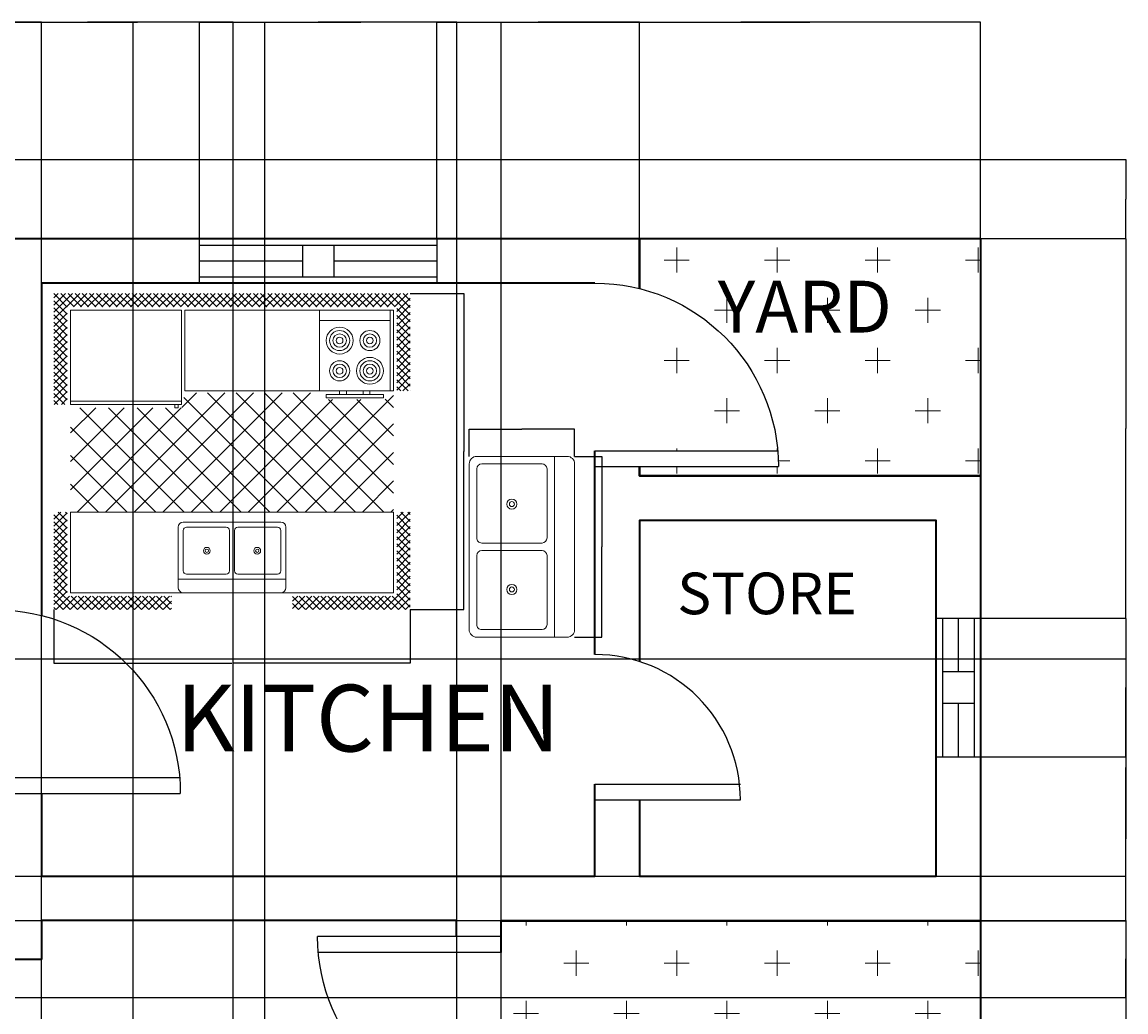
# Model space of a CAD drawing. Units: millimetres. Extents: x 19292 to 100733, y 12374 to 26974.
# Tile 18 of 24: x 31296 to 36880, y 18550 to 23556. Entities that reach past the tile are written whole.
import ezdxf

# ---------------------------------------------------------------- set-up
doc = ezdxf.new("R2010")
doc.units = ezdxf.units.MM
for name, color, linetype, lineweight in [('A-ANNO-DIMS', 2, 'Continuous', 18), ('A-AREA-IDEN', 3, 'Continuous', 25), ('A-DOOR', 4, 'Continuous', 25), ('A-FLOR-FIXT', 9, 'Continuous', 18), ('A-FLOR-PATT', 252, 'Continuous', 13), ('A-GLAZ', 3, 'Continuous', 25), ('A-WALL', 7, 'Continuous', 35)]:
    doc.layers.add(name, color=color, linetype=linetype, lineweight=lineweight)
doc.layers.add('WINDOWS', color=50, linetype='Continuous')
doc.styles.get("Standard").update_dxf_attribs({"font": 'arial.ttf'})
doc.dimstyles.get("Standard").update_dxf_attribs({"dimtxt": 0.18, "dimasz": 0.18, "dimexe": 0.18, "dimexo": 0.0625, "dimgap": 0.09, "dimtad": 0, "dimtih": 1, "dimtoh": 1, "dimdec": 4, "dimzin": 0, "dimdsep": 46, "dimtxsty": 'Standard', "dimcen": 0.09, "dimadec": 0, "dimazin": 0, "dimtfac": 1, "dimtdec": 4, "dimtofl": 0, "dimtmove": 0, "dimatfit": 3, "dimfxl": 1, "dimtolj": 1, "dimtzin": 0, "dimarcsym": 0})

# ---------------------------------------------------------------- blocks, each defined once
blk = doc.blocks.new('WW34')
at = {"layer": 'WINDOWS'}
for p, q in [((6711.3, 3446), (7411.3, 3446)), ((6981.3, 3446), (6981.3, 3286)), ((7141.3, 3446), (7141.3, 3286)), ((6711.3, 3366), (6981.3, 3366)), ((7141.3, 3366), (7411.3, 3366)), ((6711.3, 3286), (7411.3, 3286))]:
    blk.add_line(p, q, dxfattribs=at)
for points in [[(6711.3, 3478.5), (6711.3, 3253.5)], [(7411.3, 3253.5), (7411.3, 3478.5)]]:
    blk.add_lwpolyline(points, dxfattribs=at)
blk = doc.blocks.new('WW')
at = {"layer": 'WINDOWS'}
for p, q in [((-5183.9, -4940.9), (-3983.9, -4940.9)), ((-4663.9, -4940.9), (-4663.9, -5100.9)), ((-4503.9, -4940.9), (-4503.9, -5100.9)), ((-4503.9, -4940.9), (-4503.9, -5100.9)), ((-5183.9, -5020.9), (-4663.9, -5020.9)), ((-4503.9, -5020.9), (-3983.9, -5020.9)), ((-5183.9, -5100.9), (-3983.9, -5100.9))]:
    blk.add_line(p, q, dxfattribs=at)
for points in [[(-5183.9, -5133.4), (-5183.9, -4908.4)], [(-3983.9, -4908.4), (-3983.9, -5133.4)]]:
    blk.add_lwpolyline(points, dxfattribs=at)
blk = doc.blocks.new('Kitchen Layout - 7 x 8 ft')
for p, q in [((-5, 81.32), (2.68, 89)), ((-5, 83.44), (0.56, 89)), ((-5, 85.56), (-1.56, 89)), ((-5, 87.68), (-3.68, 89)), ((-1, 84.97), (-5, 88.97)), ((1.09, 85), (-2.91, 89)), ((3.21, 85), (-0.79, 89)), ((0.81, 85), (4.81, 89)), ((5.34, 85), (1.34, 89)), ((2.93, 85), (6.93, 89)), ((7.46, 85), (3.46, 89)), ((5.05, 85), (9.05, 89)), ((9.58, 85), (5.58, 89)), ((7.17, 85), (11.17, 89)), ((11.7, 85), (7.7, 89)), ((9.29, 85), (13.29, 89)), ((13.82, 85), (9.82, 89)), ((11.41, 85), (15.41, 89)), ((15.94, 85), (11.94, 89)), ((13.53, 85), (17.53, 89)), ((18.06, 85), (14.06, 89)), ((15.65, 85), (19.65, 89)), ((20.18, 85), (16.18, 89)), ((17.78, 85), (21.78, 89)), ((22.31, 85), (18.31, 89)), ((19.9, 85), (23.9, 89)), ((24.43, 85), (20.43, 89)), ((22.02, 85), (26.02, 89)), ((26.55, 85), (22.55, 89)), ((24.14, 85), (28.14, 89)), ((28.67, 85), (24.67, 89)), ((26.26, 85), (30.26, 89)), ((30.79, 85), (26.79, 89)), ((28.38, 85), (32.38, 89)), ((32.91, 85), (28.91, 89)), ((30.5, 85), (34.5, 89)), ((35.03, 85), (31.03, 89)), ((32.63, 85), (36.63, 89)), ((37.16, 85), (33.16, 89)), ((34.75, 85), (38.75, 89)), ((39.28, 85), (35.28, 89)), ((36.87, 85), (40.87, 89)), ((41.4, 85), (37.4, 89)), ((38.99, 85), (42.99, 89)), ((43.52, 85), (39.52, 89)), ((41.11, 85), (45.11, 89)), ((45.64, 85), (41.64, 89)), ((43.23, 85), (47.23, 89)), ((47.76, 85), (43.76, 89)), ((45.35, 85), (49.35, 89)), ((49.88, 85), (45.88, 89)), ((47.47, 85), (51.47, 89)), ((52, 85), (48, 89)), ((49.6, 85), (53.6, 89)), ((54.13, 85), (50.13, 89)), ((51.72, 85), (55.72, 89)), ((56.25, 85), (52.25, 89)), ((53.84, 85), (57.84, 89)), ((58.37, 85), (54.37, 89)), ((55.96, 85), (59.96, 89)), ((60.49, 85), (56.49, 89)), ((58.08, 85), (62.08, 89)), ((62.61, 85), (58.61, 89)), ((60.2, 85), (64.2, 89)), ((64.73, 85), (60.73, 89)), ((62.32, 85), (66.32, 89)), ((66.85, 85), (62.85, 89)), ((64.45, 85), (68.45, 89)), ((68.97, 85), (64.97, 89)), ((66.57, 85), (70.57, 89)), ((71.1, 85), (67.1, 89)), ((68.69, 85), (72.69, 89)), ((73.22, 85), (69.22, 89)), ((70.81, 85), (74.81, 89)), ((75.34, 85), (71.34, 89)), ((72.93, 85), (76.93, 89)), ((77.46, 85), (73.46, 89)), ((75.05, 85), (79.05, 89)), ((79.58, 85), (75.58, 89)), ((77.17, 85), (81.17, 89)), ((81.7, 85), (77.7, 89)), ((79.29, 85), (83.29, 89)), ((83.82, 85), (79.82, 89)), ((81.42, 85), (85.42, 89)), ((85.95, 85), (81.95, 89)), ((83.54, 85), (87.54, 89)), ((88.07, 85), (84.07, 89)), ((85.66, 85), (89.66, 89)), ((90.19, 85), (86.19, 89)), ((87.78, 85), (91.78, 89)), ((92.31, 85), (88.31, 89)), ((89.9, 85), (93.9, 89)), ((94.43, 85), (90.43, 89)), ((92.02, 85), (96.02, 89)), ((96.55, 85), (92.55, 89)), ((94.14, 85), (98.14, 89)), ((101, 82.67), (94.67, 89)), ((96.27, 85), (100.27, 89)), ((101, 84.79), (96.79, 89)), ((101, 86.92), (98.92, 89)), ((-1, 82.85), (-5, 86.85)), ((97, 83.61), (101, 87.61)), ((97, 81.49), (101, 85.49)), ((-1, 80.73), (-5, 84.73)), ((-5, 79.19), (-1, 83.19)), ((-1, 78.61), (-5, 82.61)), ((34, 84), (96, 84)), ((34, 60), (34, 84)), ((96, 84), (96, 60)), ((101, 80.55), (97, 84.55)), ((97, 79.37), (101, 83.37)), ((101, 78.43), (97, 82.43)), ((-5, 77.07), (-1, 81.07)), ((-1, 76.49), (-5, 80.49)), ((-5, 74.95), (-1, 78.95)), ((74, 81), (95, 81)), ((97, 77.25), (101, 81.25)), ((101, 76.31), (97, 80.31)), ((97, 75.13), (101, 79.13)), ((-1, 74.36), (-5, 78.36)), ((-5, 72.83), (-1, 76.83)), ((-1, 72.24), (-5, 76.24)), ((101, 74.19), (97, 78.19)), ((97, 73.01), (101, 77.01)), ((101, 72.07), (97, 76.07)), ((-5, 70.71), (-1, 74.71)), ((-1, 70.12), (-5, 74.12)), ((-5, 68.59), (-1, 72.59)), ((97, 70.89), (101, 74.89)), ((101, 69.95), (97, 73.95)), ((97, 68.76), (101, 72.76)), ((-1, 68), (-5, 72)), ((-5, 66.47), (-1, 70.47)), ((-1, 65.88), (-5, 69.88)), ((101, 67.82), (97, 71.82)), ((97, 66.64), (101, 70.64)), ((101, 65.7), (97, 69.7)), ((-5, 64.35), (-1, 68.35)), ((-1, 63.76), (-5, 67.76)), ((-5, 62.22), (-1, 66.22)), ((97, 64.52), (101, 68.52)), ((101, 63.58), (97, 67.58)), ((97, 62.4), (101, 66.4)), ((-1, 61.64), (-5, 65.64)), ((-5, 60.1), (-1, 64.1)), ((-1, 59.52), (-5, 63.52)), ((101, 61.46), (97, 65.46)), ((97, 60.28), (101, 64.28)), ((100.34, 60), (97, 63.34)), ((-5, 57.98), (-1, 61.98)), ((-1, 57.39), (-5, 61.39)), ((-1.73, 56), (-5, 59.27)), ((-4.86, 56), (-1, 59.86)), ((10.4, 24), (45.9, 59.5)), ((18.88, 24), (54.38, 59.5)), ((27.37, 24), (62.87, 59.5)), ((33.03, 55.11), (37.41, 59.5)), ((96, 60), (34, 60)), ((35.85, 24), (71.35, 59.5)), ((76.2, 24), (40.7, 59.5)), ((84.68, 24), (49.18, 59.5)), ((93.17, 24), (57.67, 59.5)), ((96, 29.65), (66.15, 59.5)), ((80, 60), (80, 59)), ((82, 59), (82, 60)), ((87, 59), (87, 60)), ((89, 60), (89, 59)), ((98.22, 60), (97, 61.22)), ((98.84, 60), (101, 62.16)), ((100.96, 60), (101, 60.04)), ((-3.85, 56), (-5, 57.15)), ((-2.74, 56), (-1, 57.74)), ((0, 57), (33, 57)), ((31, 55), (31, 56)), ((32, 56), (32, 55)), ((67.71, 24), (33.68, 58.04)), ((44.34, 24), (77.84, 57.5)), ((52.82, 24), (86.32, 57.5)), ((61.31, 24), (96, 58.69)), ((96, 38.14), (76.64, 57.5)), ((96, 46.63), (85.13, 57.5)), ((96, 55.11), (93.57, 57.54)), ((0, 30.57), (24.43, 55)), ((0, 39.06), (15.94, 55)), ((0, 47.54), (7.46, 55)), ((1.91, 24), (32.91, 55)), ((33.77, 24), (2.77, 55)), ((42.26, 24), (11.26, 55)), ((50.74, 24), (19.74, 55)), ((59.23, 24), (28.23, 55)), ((32, 55), (31, 55)), ((25.29, 24), (0, 49.29)), ((69.79, 24), (96, 50.21)), ((16.8, 24), (0, 40.8)), ((78.28, 24), (96, 41.72)), ((86.76, 24), (96, 33.24)), ((8.32, 24), (0, 32.32)), ((-5, 21.92), (-2.92, 24)), ((-5, 19.8), (-1, 23.8)), ((-1, 19.21), (-5, 23.21)), ((-1, 21.33), (-3.67, 24)), ((-1, 23.45), (-1.55, 24)), ((0, 24), (96, 24)), ((0, 0), (0, 24)), ((95.25, 24), (96, 24.75)), ((96, 24), (96, 0)), ((97, 22.1), (98.9, 24)), ((97, 19.97), (101, 23.97)), ((101, 19.03), (97, 23.03)), ((101, 21.16), (98.16, 24)), ((101, 23.28), (100.28, 24)), ((-5, 17.68), (-1, 21.68)), ((-1, 17.09), (-5, 21.09)), ((97, 17.85), (101, 21.85)), ((101, 16.91), (97, 20.91)), ((97, 15.73), (101, 19.73)), ((-5, 15.55), (-1, 19.55)), ((-1, 14.97), (-5, 18.97)), ((-5, 13.43), (-1, 17.43)), ((-1, 12.85), (-5, 16.85)), ((47.25, 6.5), (47.25, 18.5)), ((48.75, 18.5), (48.75, 6.5)), ((101, 14.79), (97, 18.79)), ((97, 13.61), (101, 17.61)), ((101, 12.67), (97, 16.67)), ((-5, 11.31), (-1, 15.31)), ((-1, 10.73), (-5, 14.73)), ((-5, 9.19), (-1, 13.19)), ((97, 11.49), (101, 15.49)), ((101, 10.55), (97, 14.55)), ((97, 9.37), (101, 13.37)), ((-1, 8.6), (-5, 12.6)), ((-5, 7.07), (-1, 11.07)), ((-1, 6.48), (-5, 10.48)), ((101, 8.43), (97, 12.43)), ((97, 7.25), (101, 11.25)), ((101, 6.31), (97, 10.31)), ((-5, 4.95), (-1, 8.95)), ((-1, 4.36), (-5, 8.36)), ((-5, 2.83), (-1, 6.83)), ((97, 5.12), (101, 9.12)), ((101, 4.18), (97, 8.18)), ((97, 3), (101, 7)), ((-1, 2.24), (-5, 6.24)), ((-5, 0.71), (-1, 4.71)), ((-1, 0.12), (-5, 4.12)), ((64, 4), (32, 4)), ((101, 2.06), (97, 6.06)), ((97, 0.88), (101, 4.88)), ((101, -0.06), (97, 3.94)), ((-5, -1.42), (-1, 2.58)), ((2, -5), (-5, 2)), ((-5, -3.54), (-1, 0.46)), ((96, 0), (0, 0)), ((93.24, -5), (101, 2.76)), ((95.36, -5), (101, 0.64)), ((101, -2.18), (97, 1.82)), ((-0.12, -5), (-5, -0.12)), ((-2.25, -5), (-5, -2.25)), ((-4.34, -5), (-0.34, -1)), ((-2.22, -5), (1.78, -1)), ((-0.1, -5), (3.9, -1)), ((4.12, -5), (0.12, -1)), ((2.02, -5), (6.02, -1)), ((6.24, -5), (2.24, -1)), ((4.14, -5), (8.14, -1)), ((8.36, -5), (4.36, -1)), ((6.27, -5), (10.27, -1)), ((10.48, -5), (6.48, -1)), ((8.39, -5), (12.39, -1)), ((12.6, -5), (8.6, -1)), ((10.51, -5), (14.51, -1)), ((14.73, -5), (10.73, -1)), ((12.63, -5), (16.63, -1)), ((16.85, -5), (12.85, -1)), ((14.75, -5), (18.75, -1)), ((18.97, -5), (14.97, -1)), ((16.87, -5), (20.87, -1)), ((21.09, -5), (17.09, -1)), ((18.99, -5), (22.99, -1)), ((23.21, -5), (19.21, -1)), ((21.11, -5), (25.11, -1)), ((25.33, -5), (21.33, -1)), ((23.24, -5), (27.24, -1)), ((27.45, -5), (23.45, -1)), ((25.36, -5), (29.36, -1)), ((29.57, -5), (25.57, -1)), ((27.48, -5), (30, -2.48)), ((30, -3.3), (27.7, -1)), ((30, -1.18), (29.82, -1)), ((66, -2.54), (67.54, -1)), ((66, -4.66), (69.66, -1)), ((69.88, -5), (66, -1.12)), ((67.76, -5), (66, -3.24)), ((67.78, -5), (71.78, -1)), ((72, -5), (68, -1)), ((69.9, -5), (73.9, -1)), ((74.12, -5), (70.12, -1)), ((72.03, -5), (76.03, -1)), ((76.24, -5), (72.24, -1)), ((74.15, -5), (78.15, -1)), ((78.36, -5), (74.36, -1)), ((76.27, -5), (80.27, -1)), ((80.49, -5), (76.49, -1)), ((78.39, -5), (82.39, -1)), ((82.61, -5), (78.61, -1)), ((80.51, -5), (84.51, -1)), ((84.73, -5), (80.73, -1)), ((82.63, -5), (86.63, -1)), ((86.85, -5), (82.85, -1)), ((84.75, -5), (88.75, -1)), ((88.97, -5), (84.97, -1)), ((86.88, -5), (90.88, -1)), ((91.09, -5), (87.09, -1)), ((89, -5), (93, -1)), ((93.21, -5), (89.21, -1)), ((91.12, -5), (95.12, -1)), ((95.34, -5), (91.34, -1)), ((97.46, -5), (93.46, -1)), ((99.58, -5), (95.58, -1)), ((101, -4.3), (97, -0.3)), ((97.48, -5), (101, -1.48)), ((-4.37, -5), (-5, -4.37)), ((29.6, -5), (30, -4.6)), ((99.6, -5), (101, -3.6))]:
    blk.add_line(p, q)
for points in [[(0, 56), (0, 84), (33, 84), (33, 56)], [(74, 60), (74, 84), (95, 84), (95, 60)], [(76, 58), (76, 59), (93, 59), (93, 58)]]:
    blk.add_lwpolyline(points, close=True)
for points in [[(33.5, 21), (62.5, 21)], [(32, 1.5), (32, 19.5)], [(33.5, 6.5), (33.5, 18.5)], [(34.5, 19.5), (46.25, 19.5)], [(49.75, 19.5), (61.5, 19.5)], [(62.5, 18.5), (62.5, 6.5)], [(64, 19.5), (64, 1.5)], [(46.25, 5.5), (34.5, 5.5)], [(61.5, 5.5), (49.75, 5.5)], [(62.5, 0), (33.5, 0)]]:
    blk.add_lwpolyline(points)
for centre, radius in [((80, 75), 4), ((80, 75), 3), ((80, 75), 2), ((80, 75), 1), ((89, 75), 3), ((89, 75), 2), ((89, 75), 1), ((80, 66), 3), ((89, 66), 4), ((89, 66), 3), ((80, 66), 2), ((80, 66), 1), ((89, 66), 2), ((89, 66), 1), ((40.5, 12.5), 1), ((55.5, 12.5), 1), ((40.5, 12.5), 0.5), ((55.5, 12.5), 0.5)]:
    blk.add_circle(centre, radius)
for centre, radius, start, end in [((33.5, 19.5), 1.5, 90, 180), ((62.5, 19.5), 1.5, 0, 90), ((34.5, 18.5), 1, 90, 180), ((46.25, 18.5), 1, 0, 90), ((49.75, 18.5), 1, 90, 180), ((61.5, 18.5), 1, 0, 90), ((34.5, 6.5), 1, 180, 270), ((46.25, 6.5), 1, 270, 0), ((49.75, 6.5), 1, 180, 270), ((61.5, 6.5), 1, 270, 0), ((33.5, 1.5), 1.5, 180, 270), ((62.5, 1.5), 1.5, 270, 0)]:
    blk.add_arc(centre, radius, start, end)
blk = doc.blocks.new('Sink-double - 36 in top')
for p, q in [((-18, -4), (18, -4)), ((-0.75, -18.5), (-0.75, -6.5)), ((0.75, -6.5), (0.75, -18.5))]:
    blk.add_line(p, q)
for points in [[(-16.5, 0), (16.5, 0)], [(-18, -19.5), (-18, -1.5)], [(18, -1.5), (18, -19.5)], [(-16.5, -18.5), (-16.5, -6.5)], [(-15.5, -5.5), (-1.75, -5.5)], [(1.75, -5.5), (15.5, -5.5)], [(16.5, -6.5), (16.5, -18.5)], [(-1.75, -19.5), (-15.5, -19.5)], [(15.5, -19.5), (1.75, -19.5)], [(16.5, -21), (-16.5, -21)]]:
    blk.add_lwpolyline(points)
for centre, radius in [((-8.5, -12.5), 1), ((-8.5, -12.5), 0.5), ((8.5, -12.5), 1), ((8.5, -12.5), 0.5)]:
    blk.add_circle(centre, radius)
for centre, radius, start, end in [((-16.5, -1.5), 1.5, 90, 180), ((16.5, -1.5), 1.5, 0, 90), ((-15.5, -6.5), 1, 90, 180), ((-1.75, -6.5), 1, 0, 90), ((1.75, -6.5), 1, 90, 180), ((15.5, -6.5), 1, 0, 90), ((-16.5, -19.5), 1.5, 180, 270), ((-15.5, -18.5), 1, 180, 270), ((-1.75, -18.5), 1, 270, 0), ((1.75, -18.5), 1, 180, 270), ((15.5, -18.5), 1, 270, 0), ((16.5, -19.5), 1.5, 270, 0)]:
    blk.add_arc(centre, radius, start, end)
blk = doc.blocks.new('DOOR-900')
for p, q in [((927.7, 80), (0, 80)), ((927.7, 0), (927.7, 80)), ((927.7, 0), (927.7, 80)), ((927.7, 0), (0, 0))]:
    blk.add_line(p, q)
blk.add_arc((927.7, 0), 927.7, 90, 180)
blk = doc.blocks.new('DOOR-SWING-900')
blk.add_line((927.7, 927.7), (927.7, 0))
blk.add_arc((927.7, 927.7), 927.7, 180, 270)
blk = doc.blocks.new('DOOR-SWING-750')
blk.add_line((0, 0), (735.3, 0))
blk.add_arc((0, 0), 735.3, 0, 90)
blk = doc.blocks.new('*D52')
at = {"layer": 'A-ANNO-DIMS', "color": 0, "lineweight": -2, "transparency": 16777216}
for p, q in [((31457.2, 20584.7), (31457.2, 20314.2)), ((33259.7, 20584.7), (33259.7, 20314.2)), ((31457.4, 20314.4), (32356.9, 20314.4)), ((33259.5, 20314.4), (32360.1, 20314.4))]:
    blk.add_line(p, q, dxfattribs=at)
at = {"layer": 'A-ANNO-DIMS', "color": 0, "transparency": 16777216}
for points in [[(31457.4, 20314.5), (31457.4, 20314.4), (31457.2, 20314.4)], [(33259.5, 20314.5), (33259.5, 20314.4), (33259.7, 20314.4)]]:
    blk.add_solid(points, dxfattribs=at)
at = {"layer": 'Defpoints', "color": 0, "transparency": 16777216}
for p in [(31457.2, 20584.8), (33259.7, 20584.8), (33259.7, 20314.4)]:
    blk.add_point(p, dxfattribs=at)
at = {"layer": 'A-ANNO-DIMS', "color": 0, "transparency": 16777216, "insert": (32358.5, 20314.4), "char_height": 0.18, "attachment_point": 5}
blk.add_mtext('\\A1;KITCHEN COUNTER 1803', dxfattribs=at)
blk = doc.blocks.new('*D53')
at = {"layer": 'A-ANNO-DIMS', "color": 0, "lineweight": -2, "transparency": 16777216}
for p, q in [((33259.8, 22183.3), (33530.3, 22183.3)), ((33530.1, 22183.1), (33530.1, 21384.2)), ((33530.1, 20585), (33530.1, 21383.9)), ((33259.8, 20584.8), (33530.3, 20584.8))]:
    blk.add_line(p, q, dxfattribs=at)
at = {"layer": 'A-ANNO-DIMS', "color": 0, "transparency": 16777216}
for points in [[(33530.1, 22183.1), (33530.1, 22183.1), (33530.1, 22183.3)], [(33530.1, 20585), (33530.1, 20585), (33530.1, 20584.8)]]:
    blk.add_solid(points, dxfattribs=at)
at = {"layer": 'Defpoints', "color": 0, "transparency": 16777216}
for p in [(33259.7, 22183.3), (33530.1, 22183.3), (33259.7, 20584.8)]:
    blk.add_point(p, dxfattribs=at)
at = {"layer": 'A-ANNO-DIMS', "color": 0, "transparency": 16777216, "insert": (33530.1, 21384), "char_height": 0.18, "attachment_point": 5}
blk.add_mtext('\\A1;1598', dxfattribs=at)
blk = doc.blocks.new('*D54')
at = {"layer": 'A-ANNO-DIMS', "color": 0, "lineweight": -2, "transparency": 16777216}
for p, q in [((34091.3, 21359.4), (34228.6, 21359.4)), ((34228.4, 21359.2), (34228.4, 20902.4)), ((34228.4, 20445.2), (34228.4, 20902)), ((34091.3, 20445), (34228.6, 20445))]:
    blk.add_line(p, q, dxfattribs=at)
at = {"layer": 'A-ANNO-DIMS', "color": 0, "transparency": 16777216}
for points in [[(34228.4, 21359.2), (34228.5, 21359.2), (34228.4, 21359.4)], [(34228.4, 20445.2), (34228.5, 20445.2), (34228.4, 20445)]]:
    blk.add_solid(points, dxfattribs=at)
at = {"layer": 'Defpoints', "color": 0, "transparency": 16777216}
for p in [(34091.3, 21359.4), (34091.3, 20445), (34228.4, 20445)]:
    blk.add_point(p, dxfattribs=at)
at = {"layer": 'A-ANNO-DIMS', "color": 0, "transparency": 16777216, "insert": (34228.4, 20902.2), "char_height": 0.18, "attachment_point": 5}
blk.add_mtext('\\A1;DOUBLE SINK 914', dxfattribs=at)
blk = doc.blocks.new('*D55')
at = {"layer": 'A-ANNO-DIMS', "color": 0, "lineweight": -2, "transparency": 16777216}
for p, q in [((33557.9, 21359.5), (33557.9, 21496.8)), ((33558, 21496.6), (33824.3, 21496.6)), ((34091.1, 21496.6), (33824.9, 21496.6)), ((34091.3, 21359.5), (34091.3, 21496.8))]:
    blk.add_line(p, q, dxfattribs=at)
at = {"layer": 'A-ANNO-DIMS', "color": 0, "transparency": 16777216}
for points in [[(33558, 21496.6), (33558, 21496.5), (33557.9, 21496.6)], [(34091.1, 21496.6), (34091.1, 21496.5), (34091.3, 21496.6)]]:
    blk.add_solid(points, dxfattribs=at)
at = {"layer": 'Defpoints', "color": 0, "transparency": 16777216}
for p in [(34091.3, 21496.6), (33557.9, 21359.4), (34091.3, 21359.4)]:
    blk.add_point(p, dxfattribs=at)
at = {"layer": 'A-ANNO-DIMS', "color": 0, "transparency": 16777216, "insert": (33824.6, 21496.6), "char_height": 0.18, "attachment_point": 5}
blk.add_mtext('\\A1;533', dxfattribs=at)
blk = doc.blocks.new('*D63')
at = {"layer": 'A-ANNO-DIMS', "color": 0, "lineweight": -2, "transparency": 16777216}
for p, q in [((31169.1, 22460.8), (31169.1, 23555.9)), ((31169.3, 23555.7), (31681.3, 23555.7)), ((32194, 23555.7), (31682, 23555.7)), ((32194.1, 22460.8), (32194.1, 23555.9))]:
    blk.add_line(p, q, dxfattribs=at)
at = {"layer": 'A-ANNO-DIMS', "color": 0, "transparency": 16777216}
for points in [[(31169.3, 23555.8), (31169.3, 23555.7), (31169.1, 23555.7)], [(32194, 23555.8), (32194, 23555.7), (32194.1, 23555.7)]]:
    blk.add_solid(points, dxfattribs=at)
at = {"layer": 'Defpoints', "color": 0, "transparency": 16777216}
for p in [(32194.1, 23555.7), (31169.1, 22460.7), (32194.1, 22460.7)]:
    blk.add_point(p, dxfattribs=at)
at = {"layer": 'A-ANNO-DIMS', "color": 0, "transparency": 16777216, "insert": (31681.6, 23555.7), "char_height": 0.18, "attachment_point": 5}
blk.add_mtext('\\A1;1025', dxfattribs=at)
blk = doc.blocks.new('*D64')
at = {"layer": 'A-ANNO-DIMS', "color": 0, "lineweight": -2, "transparency": 16777216}
for p, q in [((32194.1, 22460.8), (32194.1, 23555.9)), ((32194.3, 23555.7), (32793.8, 23555.7)), ((33394, 23555.7), (32794.5, 23555.7)), ((33394.1, 22460.8), (33394.1, 23555.9))]:
    blk.add_line(p, q, dxfattribs=at)
at = {"layer": 'A-ANNO-DIMS', "color": 0, "transparency": 16777216}
for points in [[(32194.3, 23555.8), (32194.3, 23555.7), (32194.1, 23555.7)], [(33394, 23555.8), (33394, 23555.7), (33394.1, 23555.7)]]:
    blk.add_solid(points, dxfattribs=at)
at = {"layer": 'Defpoints', "color": 0, "transparency": 16777216}
for p in [(33394.1, 23555.7), (32194.1, 22460.7), (33394.1, 22460.7)]:
    blk.add_point(p, dxfattribs=at)
at = {"layer": 'A-ANNO-DIMS', "color": 0, "transparency": 16777216, "insert": (32794.1, 23555.7), "char_height": 0.18, "attachment_point": 5}
blk.add_mtext('\\A1;1200', dxfattribs=at)
blk = doc.blocks.new('*D65')
at = {"layer": 'A-ANNO-DIMS', "color": 0, "lineweight": -2, "transparency": 16777216}
for p, q in [((33394.1, 22460.8), (33394.1, 23555.9)), ((33394.3, 23555.7), (33906.3, 23555.7)), ((34419, 23555.7), (33907, 23555.7)), ((34419.1, 22460.8), (34419.1, 23555.9))]:
    blk.add_line(p, q, dxfattribs=at)
at = {"layer": 'A-ANNO-DIMS', "color": 0, "transparency": 16777216}
for points in [[(33394.3, 23555.8), (33394.3, 23555.7), (33394.1, 23555.7)], [(34419, 23555.8), (34419, 23555.7), (34419.1, 23555.7)]]:
    blk.add_solid(points, dxfattribs=at)
at = {"layer": 'Defpoints', "color": 0, "transparency": 16777216}
for p in [(34419.1, 23555.7), (33394.1, 22460.7), (34419.1, 22460.7)]:
    blk.add_point(p, dxfattribs=at)
at = {"layer": 'A-ANNO-DIMS', "color": 0, "transparency": 16777216, "insert": (33906.6, 23555.7), "char_height": 0.18, "attachment_point": 5}
blk.add_mtext('\\A1;1025', dxfattribs=at)
blk = doc.blocks.new('*D66')
at = {"layer": 'A-ANNO-DIMS', "color": 0, "lineweight": -2, "transparency": 16777216}
for p, q in [((34419.1, 22460.8), (34419.1, 23555.9)), ((34419.3, 23555.7), (35281.3, 23555.7)), ((36144, 23555.7), (35282, 23555.7)), ((36144.1, 22460.8), (36144.1, 23555.9))]:
    blk.add_line(p, q, dxfattribs=at)
at = {"layer": 'A-ANNO-DIMS', "color": 0, "transparency": 16777216}
for points in [[(34419.3, 23555.8), (34419.3, 23555.7), (34419.1, 23555.7)], [(36144, 23555.8), (36144, 23555.7), (36144.1, 23555.7)]]:
    blk.add_solid(points, dxfattribs=at)
at = {"layer": 'Defpoints', "color": 0, "transparency": 16777216}
for p in [(36144.1, 23555.7), (34419.1, 22460.7), (36144.1, 22460.7)]:
    blk.add_point(p, dxfattribs=at)
at = {"layer": 'A-ANNO-DIMS', "color": 0, "transparency": 16777216, "insert": (35281.6, 23555.7), "char_height": 0.18, "attachment_point": 5}
blk.add_mtext('\\A1;1725', dxfattribs=at)
blk = doc.blocks.new('*D68')
at = {"layer": 'A-ANNO-DIMS', "color": 0, "lineweight": -2, "transparency": 16777216}
for p, q in [((22919.2, 20335.7), (36879.3, 20335.7)), ((36879.2, 20335.5), (36879.2, 19785.9)), ((36879.2, 19235.9), (36879.2, 19785.5)), ((22919.2, 19235.7), (36879.3, 19235.7))]:
    blk.add_line(p, q, dxfattribs=at)
at = {"layer": 'A-ANNO-DIMS', "color": 0, "transparency": 16777216}
for points in [[(36879.1, 20335.5), (36879.2, 20335.5), (36879.2, 20335.7)], [(36879.1, 19235.9), (36879.2, 19235.9), (36879.2, 19235.7)]]:
    blk.add_solid(points, dxfattribs=at)
at = {"layer": 'Defpoints', "color": 0, "transparency": 16777216}
for p in [(22919.1, 20335.7), (22919.1, 19235.7), (36879.2, 19235.7)]:
    blk.add_point(p, dxfattribs=at)
at = {"layer": 'A-ANNO-DIMS', "color": 0, "transparency": 16777216, "insert": (36879.2, 19785.7), "char_height": 0.18, "attachment_point": 5}
blk.add_mtext('\\A1;1100', dxfattribs=at)
blk = doc.blocks.new('*D69')
at = {"layer": 'A-ANNO-DIMS', "color": 0, "lineweight": -2, "transparency": 16777216}
for p, q in [((23573.9, 19012.7), (36879.3, 19012.7)), ((36879.2, 19012.6), (36879.2, 18818)), ((36879.2, 18623), (36879.2, 18817.6)), ((23573.9, 18622.9), (36879.3, 18622.9))]:
    blk.add_line(p, q, dxfattribs=at)
at = {"layer": 'A-ANNO-DIMS', "color": 0, "transparency": 16777216}
for points in [[(36879.1, 19012.6), (36879.2, 19012.6), (36879.2, 19012.7)], [(36879.1, 18623), (36879.2, 18623), (36879.2, 18622.9)]]:
    blk.add_solid(points, dxfattribs=at)
at = {"layer": 'Defpoints', "color": 0, "transparency": 16777216}
for p in [(23573.8, 19012.7), (23573.8, 18622.9), (36879.2, 18622.9)]:
    blk.add_point(p, dxfattribs=at)
at = {"layer": 'A-ANNO-DIMS', "color": 0, "transparency": 16777216, "insert": (36879.2, 18817.8), "char_height": 0.18, "attachment_point": 5}
blk.add_mtext('\\A1;389.9', dxfattribs=at)
blk = doc.blocks.new('*D74')
at = {"layer": 'A-ANNO-DIMS', "color": 0, "lineweight": -2, "transparency": 16777216}
for p, q in [((36144.2, 19010.7), (36879.3, 19010.7)), ((36879.2, 19010.5), (36879.2, 17498.4)), ((36879.2, 15985.9), (36879.2, 17498)), ((36144.2, 15985.7), (36879.3, 15985.7))]:
    blk.add_line(p, q, dxfattribs=at)
at = {"layer": 'A-ANNO-DIMS', "color": 0, "transparency": 16777216}
for points in [[(36879.1, 19010.5), (36879.2, 19010.5), (36879.2, 19010.7)], [(36879.1, 15985.9), (36879.2, 15985.9), (36879.2, 15985.7)]]:
    blk.add_solid(points, dxfattribs=at)
at = {"layer": 'Defpoints', "color": 0, "transparency": 16777216}
for p in [(36144.2, 19010.7), (36879.2, 19010.7), (36144.2, 15985.7)]:
    blk.add_point(p, dxfattribs=at)
at = {"layer": 'A-ANNO-DIMS', "color": 0, "transparency": 16777216, "insert": (36879.2, 17498.2), "char_height": 0.18, "attachment_point": 5}
blk.add_mtext('\\A1;3025', dxfattribs=at)
blk = doc.blocks.new('*D75')
at = {"layer": 'A-ANNO-DIMS', "color": 0, "lineweight": -2, "transparency": 16777216}
for p, q in [((36144.2, 19840.4), (36879.3, 19840.4)), ((36879.2, 19840.2), (36879.2, 19425.7)), ((36879.2, 19010.9), (36879.2, 19425.4)), ((36144.2, 19010.7), (36879.3, 19010.7))]:
    blk.add_line(p, q, dxfattribs=at)
at = {"layer": 'A-ANNO-DIMS', "color": 0, "transparency": 16777216}
for points in [[(36879.1, 19840.2), (36879.2, 19840.2), (36879.2, 19840.4)], [(36879.1, 19010.9), (36879.2, 19010.9), (36879.2, 19010.7)]]:
    blk.add_solid(points, dxfattribs=at)
at = {"layer": 'Defpoints', "color": 0, "transparency": 16777216}
for p in [(36144.1, 19840.4), (36879.2, 19840.4), (36144.2, 19010.7)]:
    blk.add_point(p, dxfattribs=at)
at = {"layer": 'A-ANNO-DIMS', "color": 0, "transparency": 16777216, "insert": (36879.2, 19425.6), "char_height": 0.18, "attachment_point": 5}
blk.add_mtext('\\A1;829.7', dxfattribs=at)
blk = doc.blocks.new('*D76')
at = {"layer": 'A-ANNO-DIMS', "color": 0, "lineweight": -2, "transparency": 16777216}
for p, q in [((36144.2, 20540.4), (36879.3, 20540.4)), ((36879.2, 20540.2), (36879.2, 20190.6)), ((36879.2, 19840.6), (36879.2, 20190.2)), ((36144.2, 19840.4), (36879.3, 19840.4))]:
    blk.add_line(p, q, dxfattribs=at)
at = {"layer": 'A-ANNO-DIMS', "color": 0, "transparency": 16777216}
for points in [[(36879.1, 20540.2), (36879.2, 20540.2), (36879.2, 20540.4)], [(36879.1, 19840.6), (36879.2, 19840.6), (36879.2, 19840.4)]]:
    blk.add_solid(points, dxfattribs=at)
at = {"layer": 'Defpoints', "color": 0, "transparency": 16777216}
for p in [(36144.1, 20540.4), (36879.2, 20540.4), (36144.1, 19840.4)]:
    blk.add_point(p, dxfattribs=at)
at = {"layer": 'A-ANNO-DIMS', "color": 0, "transparency": 16777216, "insert": (36879.2, 20190.4), "char_height": 0.18, "attachment_point": 5}
blk.add_mtext('\\A1;700', dxfattribs=at)
blk = doc.blocks.new('*D77')
at = {"layer": 'A-ANNO-DIMS', "color": 0, "lineweight": -2, "transparency": 16777216}
for p, q in [((36144.2, 22460.7), (36879.3, 22460.7)), ((36879.2, 22460.5), (36879.2, 21500.7)), ((36879.2, 20540.6), (36879.2, 21500.4)), ((36144.2, 20540.4), (36879.3, 20540.4))]:
    blk.add_line(p, q, dxfattribs=at)
at = {"layer": 'A-ANNO-DIMS', "color": 0, "transparency": 16777216}
for points in [[(36879.1, 22460.5), (36879.2, 22460.5), (36879.2, 22460.7)], [(36879.1, 20540.6), (36879.2, 20540.6), (36879.2, 20540.4)]]:
    blk.add_solid(points, dxfattribs=at)
at = {"layer": 'Defpoints', "color": 0, "transparency": 16777216}
for p in [(36144.1, 22460.7), (36879.2, 22460.7), (36144.1, 20540.4)]:
    blk.add_point(p, dxfattribs=at)
at = {"layer": 'A-ANNO-DIMS', "color": 0, "transparency": 16777216, "insert": (36879.2, 21500.6), "char_height": 0.18, "attachment_point": 5}
blk.add_mtext('\\A1;1920.3', dxfattribs=at)
blk = doc.blocks.new('*D78')
at = {"layer": 'A-ANNO-DIMS', "color": 0, "lineweight": -2, "transparency": 16777216}
for p, q in [((28369.2, 22860.7), (36879.3, 22860.7)), ((36879.2, 22860.5), (36879.2, 22660.9)), ((36879.2, 22460.9), (36879.2, 22660.5)), ((36144.2, 22460.7), (36879.3, 22460.7))]:
    blk.add_line(p, q, dxfattribs=at)
at = {"layer": 'A-ANNO-DIMS', "color": 0, "transparency": 16777216}
for points in [[(36879.1, 22860.5), (36879.2, 22860.5), (36879.2, 22860.7)], [(36879.1, 22460.9), (36879.2, 22460.9), (36879.2, 22460.7)]]:
    blk.add_solid(points, dxfattribs=at)
at = {"layer": 'Defpoints', "color": 0, "transparency": 16777216}
for p in [(28369.1, 22860.7), (36879.2, 22860.7), (36144.1, 22460.7)]:
    blk.add_point(p, dxfattribs=at)
at = {"layer": 'A-ANNO-DIMS', "color": 0, "transparency": 16777216, "insert": (36879.2, 22660.7), "char_height": 0.18, "attachment_point": 5}
blk.add_mtext('\\A1;400', dxfattribs=at)
blk = doc.blocks.new('*D79')
at = {"layer": 'A-ANNO-DIMS', "color": 0, "lineweight": -2, "transparency": 16777216}
for p, q in [((22694.1, 22860.7), (22694.1, 12808.8)), ((36144.2, 15985.7), (36144.2, 12808.8)), ((22694.3, 12809), (29418.7, 12809)), ((36144, 12809), (29419.6, 12809))]:
    blk.add_line(p, q, dxfattribs=at)
at = {"layer": 'A-ANNO-DIMS', "color": 0, "transparency": 16777216}
for points in [[(22694.3, 12809), (22694.3, 12809), (22694.1, 12809)], [(36144, 12809), (36144, 12809), (36144.2, 12809)]]:
    blk.add_solid(points, dxfattribs=at)
at = {"layer": 'Defpoints', "color": 0, "transparency": 16777216}
for p in [(22694.1, 22860.7), (36144.2, 15985.7), (36144.2, 12809)]:
    blk.add_point(p, dxfattribs=at)
at = {"layer": 'A-ANNO-DIMS', "color": 0, "transparency": 16777216, "insert": (29419.2, 12809), "char_height": 0.18, "attachment_point": 5}
blk.add_mtext('\\A1;13450', dxfattribs=at)
blk = doc.blocks.new('*D82')
at = {"layer": 'A-ANNO-DIMS', "color": 0, "lineweight": -2, "transparency": 16777216}
for p, q in [((27198.8, 13562.8), (27198.8, 23555.9)), ((27199, 23555.7), (29296.4, 23555.7)), ((31394.6, 23555.7), (29297.2, 23555.7)), ((31394.8, 13544.1), (31394.8, 23555.9))]:
    blk.add_line(p, q, dxfattribs=at)
at = {"layer": 'A-ANNO-DIMS', "color": 0, "transparency": 16777216}
for points in [[(27199, 23555.8), (27199, 23555.7), (27198.8, 23555.7)], [(31394.6, 23555.8), (31394.6, 23555.7), (31394.8, 23555.7)]]:
    blk.add_solid(points, dxfattribs=at)
at = {"layer": 'Defpoints', "color": 0, "transparency": 16777216}
for p in [(31394.8, 23555.7), (27198.8, 13562.7), (31394.8, 13544)]:
    blk.add_point(p, dxfattribs=at)
at = {"layer": 'A-ANNO-DIMS', "color": 0, "transparency": 16777216, "insert": (29296.8, 23555.7), "char_height": 0.18, "attachment_point": 5}
blk.add_mtext('\\A1;4196', dxfattribs=at)
blk = doc.blocks.new('*D83')
at = {"layer": 'A-ANNO-DIMS', "color": 0, "lineweight": -2, "transparency": 16777216}
for p, q in [((31394.8, 15131.5), (31394.8, 23555.9)), ((31395, 23555.7), (31626.3, 23555.7)), ((31858.6, 23555.7), (31627.2, 23555.7)), ((31858.7, 15131.5), (31858.7, 23555.9))]:
    blk.add_line(p, q, dxfattribs=at)
at = {"layer": 'A-ANNO-DIMS', "color": 0, "transparency": 16777216}
for points in [[(31395, 23555.8), (31395, 23555.7), (31394.8, 23555.7)], [(31858.6, 23555.8), (31858.6, 23555.7), (31858.7, 23555.7)]]:
    blk.add_solid(points, dxfattribs=at)
at = {"layer": 'Defpoints', "color": 0, "transparency": 16777216}
for p in [(31858.7, 23555.7), (31394.8, 15131.4), (31858.7, 15131.4)]:
    blk.add_point(p, dxfattribs=at)
at = {"layer": 'A-ANNO-DIMS', "color": 0, "transparency": 16777216, "insert": (31626.8, 23555.7), "char_height": 0.18, "attachment_point": 5}
blk.add_mtext('\\A1;463.95', dxfattribs=at)
blk = doc.blocks.new('*D84')
at = {"layer": 'A-ANNO-DIMS', "color": 0, "lineweight": -2, "transparency": 16777216}
for p, q in [((33719.2, 15985.8), (33719.2, 23555.9)), ((33719.3, 23555.7), (34931.3, 23555.7)), ((36144, 23555.7), (34932, 23555.7)), ((36144.2, 15985.8), (36144.2, 23555.9))]:
    blk.add_line(p, q, dxfattribs=at)
at = {"layer": 'A-ANNO-DIMS', "color": 0, "transparency": 16777216}
for points in [[(33719.3, 23555.8), (33719.3, 23555.7), (33719.2, 23555.7)], [(36144, 23555.8), (36144, 23555.7), (36144.2, 23555.7)]]:
    blk.add_solid(points, dxfattribs=at)
at = {"layer": 'Defpoints', "color": 0, "transparency": 16777216}
for p in [(36144.2, 23555.7), (33719.2, 15985.7), (36144.2, 15985.7)]:
    blk.add_point(p, dxfattribs=at)
at = {"layer": 'A-ANNO-DIMS', "color": 0, "transparency": 16777216, "insert": (34931.7, 23555.7), "char_height": 0.18, "attachment_point": 5}
blk.add_mtext('\\A1;2425', dxfattribs=at)
blk = doc.blocks.new('*D87')
at = {"layer": 'A-ANNO-DIMS', "color": 0, "lineweight": -2, "transparency": 16777216}
for p, q in [((32524.8, 17056.5), (32524.8, 23555.9)), ((32525, 23555.7), (33009.5, 23555.7)), ((33494.6, 23555.7), (33010.1, 23555.7)), ((33494.8, 17056.5), (33494.8, 23555.9))]:
    blk.add_line(p, q, dxfattribs=at)
at = {"layer": 'A-ANNO-DIMS', "color": 0, "transparency": 16777216}
for points in [[(32525, 23555.8), (32525, 23555.7), (32524.8, 23555.7)], [(33494.6, 23555.8), (33494.6, 23555.7), (33494.8, 23555.7)]]:
    blk.add_solid(points, dxfattribs=at)
at = {"layer": 'Defpoints', "color": 0, "transparency": 16777216}
for p in [(33494.8, 23555.7), (32524.8, 17056.4), (33494.8, 17056.4)]:
    blk.add_point(p, dxfattribs=at)
at = {"layer": 'A-ANNO-DIMS', "color": 0, "transparency": 16777216, "insert": (33009.8, 23555.7), "char_height": 0.18, "attachment_point": 5}
blk.add_mtext('\\A1;970', dxfattribs=at)
blk = doc.blocks.new('*D88')
at = {"layer": 'A-ANNO-DIMS', "color": 0, "lineweight": -2, "transparency": 16777216}
for p, q in [((31394.8, 16606.5), (31394.8, 23555.9)), ((31395, 23555.7), (31879.5, 23555.7)), ((32364.6, 23555.7), (31880.1, 23555.7)), ((32364.8, 16606.5), (32364.8, 23555.9))]:
    blk.add_line(p, q, dxfattribs=at)
at = {"layer": 'A-ANNO-DIMS', "color": 0, "transparency": 16777216}
for points in [[(31395, 23555.8), (31395, 23555.7), (31394.8, 23555.7)], [(32364.6, 23555.8), (32364.6, 23555.7), (32364.8, 23555.7)]]:
    blk.add_solid(points, dxfattribs=at)
at = {"layer": 'Defpoints', "color": 0, "transparency": 16777216}
for p in [(32364.8, 23555.7), (31394.8, 16606.4), (32364.8, 16606.4)]:
    blk.add_point(p, dxfattribs=at)
at = {"layer": 'A-ANNO-DIMS', "color": 0, "transparency": 16777216, "insert": (31879.8, 23555.7), "char_height": 0.18, "attachment_point": 5}
blk.add_mtext('\\A1;970', dxfattribs=at)

msp = doc.modelspace()

# ---------------------------------------------------------------- hatches: boundary and pattern name
at = {"layer": 'A-FLOR-PATT'}
h = msp.add_hatch(dxfattribs=at)
h.set_pattern_fill('CROSS', color=256, scale=40)
h.paths.add_polyline_path([(36144.169, 19010.725), (33719.169, 19010.725), (33719.169, 18850.725), (33719.169, 18003.026), (33719.169, 15985.725), (36144.169, 15985.725)])
h.paths.add_polyline_path([(36144.132, 22460.725), (34419.132, 22460.725), (34419.132, 22208.026, -0.34415073), (35121.831, 21308.026), (34419.132, 21308.026), (34419.132, 21260.725), (36144.132, 21260.725)])
h.paths.add_polyline_path([(34419.132, 22208.026), (34419.132, 21388.026), (35118.375, 21388.026, 0.32018294)], flags=17)
h.paths.add_polyline_path([(31169.132, 22460.725), (28369.132, 22460.725), (28369.132, 21460.725), (31169.132, 21460.725)])
h.paths.add_polyline_path([(34010.406, 17316.149), (36018.156, 17316.149), (36018.156, 17722.778), (34010.406, 17722.778)], flags=24)
h.paths.add_polyline_path([(34456.896, 21920.301), (35605.434, 21920.301), (35605.434, 22313.518), (34456.896, 22313.518)], flags=25)
h.paths.add_polyline_path([(29263.068, 21823.707), (30421.489, 21823.707), (30421.489, 22034.008), (29263.068, 22034.008)], flags=24)

# ---------------------------------------------------------------- linework, layer by layer
at = {"layer": 'A-DOOR'}
for p, q in [((34194.132, 21388.026), (35121.831, 21388.026)), ((31169.132, 19735.07), (32096.831, 19735.07)), ((34194.132, 19701.87), (34929.405, 19701.87))]:
    msp.add_line(p, q, dxfattribs=at)
at = {"layer": 'A-WALL'}
msp.add_line((31394.132, 18815.368), (31198.815, 18815.368), dxfattribs=at)
for points in [[(29548.571, 14906.403), (27198.815, 14906.403), (27198.815, 13562.748), (23348.815, 13562.748), (23348.815, 19010.725), (22694.132, 19010.725), (22694.132, 22860.725), (28369.132, 22860.725), (28369.132, 21460.725), (31169.132, 21460.725), (31169.132, 22460.725), (34419.132, 22460.725), (34419.132, 22208.026)], [(34419.132, 22208.026), (34419.132, 22460.725), (36144.132, 22460.725), (36144.132, 21260.725), (34419.132, 21260.725), (34419.132, 21308.026)], [(34194.132, 22235.725), (31394.132, 22235.725), (31394.132, 20555.07)], [(34194.132, 20357.142), (34194.132, 21388.026)], [(34419.132, 21308.026), (34419.132, 21260.725), (36144.132, 21260.725), (36144.132, 19010.725), (33719.169, 19010.725)], [(34419.132, 19621.87), (34419.132, 19235.725), (35919.132, 19235.725), (35919.132, 21035.725), (34419.132, 21035.725), (34419.132, 20321.87)], [(31394.132, 19655.07), (31394.132, 19235.725), (34194.132, 19235.725), (34194.132, 19701.87)], [(33494.132, 18930.725), (33494.132, 19012.748), (31394.132, 19012.748), (31394.132, 18815.368)], [(33719.169, 18850.725), (33719.169, 19010.725), (36144.169, 19010.725), (36144.169, 15985.725), (33719.169, 15985.725), (33719.169, 18003.026)]]:
    msp.add_lwpolyline(points, dxfattribs=at)

# ---------------------------------------------------------------- block references
at = {"layer": 'A-DOOR', "extrusion": (0, 0, -1), "zscale": -1}
for name, p, rotation in [('DOOR-SWING-900', (-35121.831, 22235.725), 270), ('DOOR-SWING-900', (-32096.831, 20582.769), 269.9999999999995), ('DOOR-900', (-32791.471, 18930.725), 180)]:
    msp.add_blockref(name, p, dxfattribs=dict(at, rotation=rotation))
at = {"layer": 'A-DOOR'}
msp.add_blockref('DOOR-SWING-750', (34194.132, 19621.87), dxfattribs=at)
at = {"layer": 'A-FLOR-FIXT', "xscale": 17.00505981237103, "yscale": 17.00505981237103, "zscale": 17.00505981237103}
msp.add_blockref('Kitchen Layout - 7 x 8 ft', (31542.218, 20669.827), dxfattribs=at)
at = {"layer": 'A-FLOR-FIXT', "xscale": 25.4, "yscale": 25.4, "zscale": 25.4, "rotation": 270}
msp.add_blockref('Sink-double - 36 in top', (34091.266, 20902.217), dxfattribs=at)
at = {"layer": 'A-GLAZ'}
msp.add_blockref('WW', (37378, 27369.102), dxfattribs=at)
at = {"layer": 'A-GLAZ', "rotation": 270}
msp.add_blockref('WW34', (32665.63, 27251.666), dxfattribs=at)

# ---------------------------------------------------------------- texts
at = {"layer": 'A-AREA-IDEN'}
for s, height, p in [('YARD', 262.1447, (34815.17, 21985.837)), ('STORE', 210.5336, (34610.429, 20561.077)), ('KITCHEN', 337.4118, (32075.075, 19867.067))]:
    msp.add_text(s, height=height, dxfattribs=at).set_placement(p)

# ---------------------------------------------------------------- dimensions: what is measured, and where the dimension line sits
at = {"layer": 'A-ANNO-DIMS'}
for base, p1, p2, override, picture, middle in [((31394.799, 23555.725), (27198.815, 13562.748), (31394.799, 13543.993), {"dimdec": 0, "dimlfac": 1, "dimrnd": 0, "dimzin": 0, "dimdsep": 46, "dimlunit": 2}, '*D82', (29296.807, 23555.725)), ((32194.132, 23555.725), (31169.132, 22460.725), (32194.132, 22460.725), {"dimdec": 0, "dimlfac": 1, "dimrnd": 0, "dimzin": 0, "dimdsep": 46, "dimlunit": 2}, '*D63', (31681.632, 23555.725)), ((31858.745, 23555.725), (31394.799, 15131.403), (31858.745, 15131.403), {"dimdec": 2, "dimlfac": 1, "dimrnd": 0, "dimzin": 0, "dimdsep": 46, "dimlunit": 2}, '*D83', (31626.772, 23555.725)), ((32364.799, 23555.725), (31394.799, 16606.403), (32364.799, 16606.403), {"dimdec": 0, "dimlfac": 1, "dimrnd": 0, "dimzin": 0, "dimdsep": 46, "dimlunit": 2}, '*D88', (31879.799, 23555.725)), ((33394.132, 23555.725), (32194.132, 22460.725), (33394.132, 22460.725), {"dimdec": 0, "dimlfac": 1, "dimrnd": 0, "dimzin": 0, "dimdsep": 46, "dimlunit": 2}, '*D64', (32794.132, 23555.725)), ((33494.799, 23555.725), (32524.799, 17056.403), (33494.799, 17056.403), {"dimdec": 0, "dimlfac": 1, "dimrnd": 0, "dimzin": 0, "dimdsep": 46, "dimlunit": 2}, '*D87', (33009.799, 23555.725)), ((34419.132, 23555.725), (33394.132, 22460.725), (34419.132, 22460.725), {"dimdec": 0, "dimlfac": 1, "dimrnd": 0, "dimzin": 0, "dimdsep": 46, "dimlunit": 2}, '*D65', (33906.632, 23555.725)), ((36144.169, 23555.725), (33719.169, 15985.725), (36144.169, 15985.725), {"dimdec": 0, "dimlfac": 1, "dimrnd": 0, "dimzin": 0, "dimdsep": 46, "dimlunit": 2}, '*D84', (34931.669, 23555.725)), ((36144.132, 23555.725), (34419.132, 22460.725), (36144.132, 22460.725), {"dimdec": 0, "dimlfac": 1, "dimrnd": 0, "dimzin": 0, "dimdsep": 46, "dimlunit": 2}, '*D66', (35281.632, 23555.725)), ((36144.169, 12808.993), (22694.132, 22860.725), (36144.169, 15985.725), {"dimdec": 0, "dimlfac": 1, "dimrnd": 0, "dimzin": 0, "dimdsep": 46, "dimlunit": 2}, '*D79', (29419.151, 12808.993)), ((34091.266, 21496.577), (33557.866, 21359.417), (34091.266, 21359.417), {"dimdec": 0, "dimrnd": 0, "dimzin": 0, "dimlunit": 2}, '*D55', (33824.566, 21496.577))]:
    dim = msp.add_linear_dim(base=base, p1=p1, p2=p2, dimstyle='Standard', override=override, dxfattribs=at)
    dim.commit()
    dim.dimension.update_dxf_attribs({"geometry": picture, "text_midpoint": middle})
for base, p1, p2, override, picture, middle in [((36879.169, 22860.725), (36144.132, 22460.725), (28369.132, 22860.725), {"dimdec": 0, "dimlfac": 1, "dimrnd": 0, "dimzin": 0, "dimdsep": 46, "dimlunit": 2}, '*D78', (36879.169, 22660.725)), ((36879.169, 22460.725), (36144.132, 20540.383), (36144.132, 22460.725), {"dimdec": 1, "dimlfac": 1, "dimrnd": 0, "dimzin": 0, "dimdsep": 46, "dimlunit": 2}, '*D77', (36879.169, 21500.554)), ((33530.11, 22183.277), (33259.729, 20584.802), (33259.729, 22183.277), {"dimdec": 0, "dimrnd": 0, "dimzin": 0, "dimlunit": 2}, '*D53', (33530.11, 21384.039)), ((36879.169, 20540.383), (36144.132, 19840.383), (36144.132, 20540.383), {"dimdec": 0, "dimlfac": 1, "dimrnd": 0, "dimzin": 0, "dimdsep": 46, "dimlunit": 2}, '*D76', (36879.169, 20190.383)), ((36879.169, 19235.725), (22919.132, 20335.725), (22919.132, 19235.725), {"dimdec": 0, "dimlfac": 1, "dimrnd": 0, "dimzin": 0, "dimdsep": 46, "dimlunit": 2}, '*D68', (36879.169, 19785.725)), ((36879.169, 19840.383), (36144.169, 19010.725), (36144.132, 19840.383), {"dimdec": 1, "dimlfac": 1, "dimrnd": 0, "dimzin": 0, "dimdsep": 46, "dimlunit": 2}, '*D75', (36879.169, 19425.554)), ((36879.169, 18622.861), (23573.815, 19012.748), (23573.815, 18622.861), {"dimdec": 1, "dimlfac": 1, "dimrnd": 0, "dimzin": 0, "dimdsep": 46, "dimlunit": 2}, '*D69', (36879.169, 18817.804)), ((36879.169, 19010.725), (36144.169, 15985.725), (36144.169, 19010.725), {"dimdec": 0, "dimlfac": 1, "dimrnd": 0, "dimzin": 0, "dimdsep": 46, "dimlunit": 2}, '*D74', (36879.169, 17498.225))]:
    dim = msp.add_linear_dim(base=base, p1=p1, p2=p2, angle=90, dimstyle='Standard', override=override, dxfattribs=at)
    dim.commit()
    dim.dimension.update_dxf_attribs({"geometry": picture, "text_midpoint": middle})
dim = msp.add_linear_dim(base=(34228.426, 20445.017), p1=(34091.266, 21359.417), p2=(34091.266, 20445.017), angle=270, text='DOUBLE SINK <>', dimstyle='Standard', override={"dimdec": 0, "dimrnd": 0, "dimzin": 0, "dimlunit": 2}, dxfattribs=at)
dim.commit()
dim.dimension.update_dxf_attribs({"geometry": '*D54', "text_midpoint": (34228.426, 20902.217)})
dim = msp.add_linear_dim(base=(33259.729, 20314.421), p1=(31457.193, 20584.802), p2=(33259.729, 20584.802), text='KITCHEN COUNTER <>', dimstyle='Standard', override={"dimdec": 0, "dimrnd": 0, "dimzin": 0, "dimlunit": 2}, dxfattribs=at)
dim.commit()
dim.dimension.update_dxf_attribs({"geometry": '*D52', "text_midpoint": (32358.461, 20314.421)})

doc.saveas('drawing.dxf')
